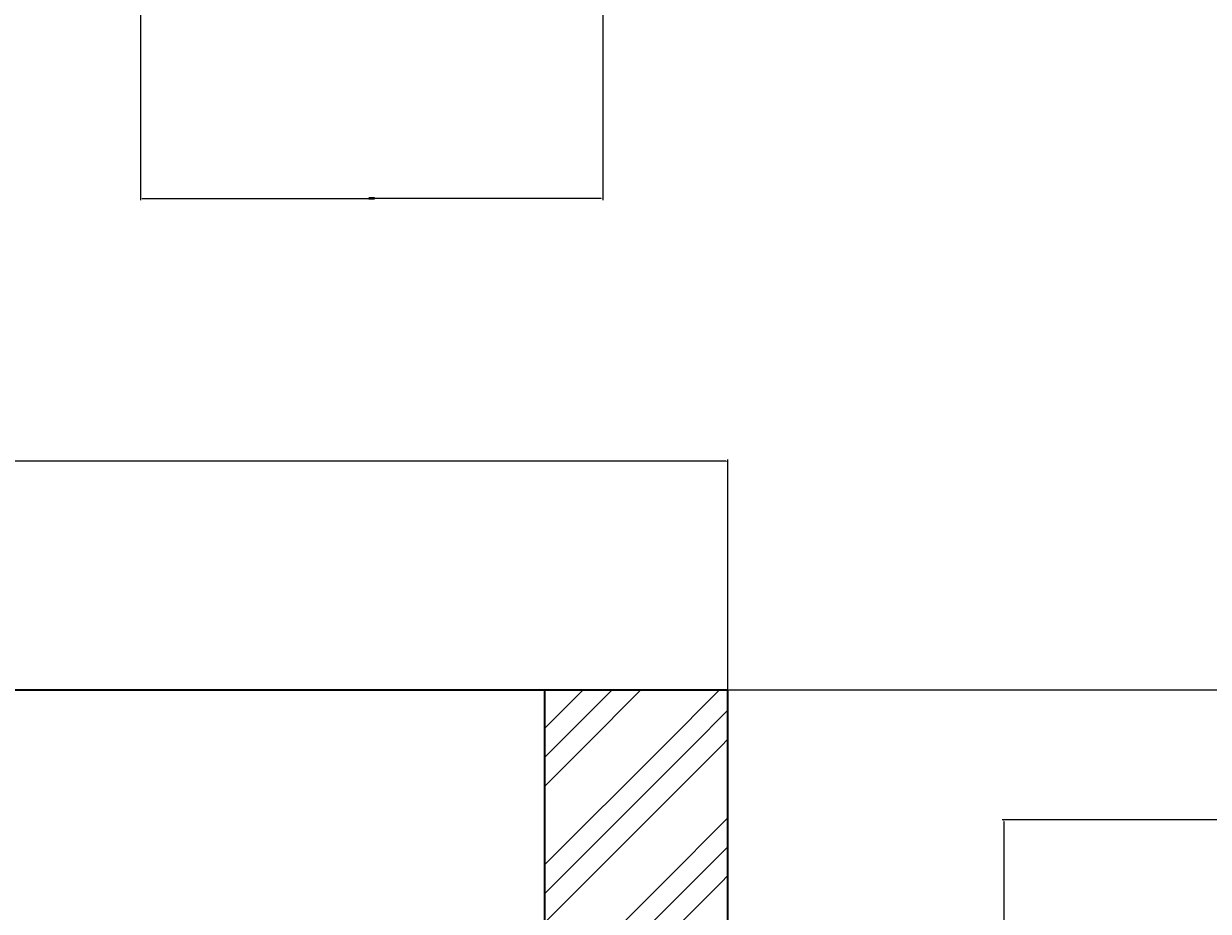
# Model space of a CAD drawing. Units: inches. Extents: x -128 to 854, y -395 to 398.
# Tile 21 of 61: x 245 to 368, y -201 to -109. Entities that reach past the tile are written whole.
import ezdxf

# ---------------------------------------------------------------- set-up
doc = ezdxf.new("R2010")
doc.units = ezdxf.units.IN
doc.header["$MEASUREMENT"] = 0
for name, color, linetype, lineweight in [('A-ANNO-DIMS', 2, 'Continuous', 18), ('A-SECT', 220, 'Continuous', 35), ('A-SECT-PATT', 8, 'Continuous', 13)]:
    doc.layers.add(name, color=color, linetype=linetype, lineweight=lineweight)
doc.styles.get("Standard").update_dxf_attribs({"font": 'arial.ttf'})
doc.dimstyles.get("Standard").update_dxf_attribs({"dimtxt": 0.18, "dimasz": 0.18, "dimexe": 0.18, "dimexo": 0.0625, "dimgap": 0.09, "dimtad": 0, "dimtih": 1, "dimtoh": 1, "dimdec": 1, "dimzin": 0, "dimdsep": 46, "dimlunit": 4, "dimtxsty": 'Standard', "dimcen": 0.09, "dimclrd": 1, "dimclre": 2, "dimclrt": 6, "dimadec": 0, "dimazin": 0, "dimtfac": 1, "dimtdec": 1, "dimtofl": 0, "dimtmove": 0, "dimatfit": 3, "dimfxl": 1, "dimtfill": 2, "dimtfillclr": 3, "dimtolj": 1, "dimtzin": 0, "dimarcsym": 0})

# ---------------------------------------------------------------- blocks, each defined once
blk = doc.blocks.new('*D114')
at = {"layer": 'A-ANNO-DIMS', "color": 2, "lineweight": -2, "transparency": 16777216}
for p, q in [((256.87, -80.32), (256.87, -127.24)), ((304.87, -80.32), (304.87, -127.24))]:
    blk.add_line(p, q, dxfattribs=at)
at = {"layer": 'A-ANNO-DIMS', "color": 1, "lineweight": -2, "transparency": 16777216}
for p, q in [((257.05, -127.06), (280.54, -127.06)), ((304.69, -127.06), (281.21, -127.06))]:
    blk.add_line(p, q, dxfattribs=at)
at = {"layer": 'A-ANNO-DIMS', "color": 1, "transparency": 16777216}
for points in [[(257.05, -127.03), (257.05, -127.09), (256.87, -127.06)], [(304.69, -127.03), (304.69, -127.09), (304.87, -127.06)]]:
    blk.add_solid(points, dxfattribs=at)
at = {"layer": 'Defpoints', "color": 0, "transparency": 16777216}
for p in [(256.87, -80.26), (304.87, -80.26), (256.87, -127.06)]:
    blk.add_point(p, dxfattribs=at)
at = {"layer": 'A-ANNO-DIMS', "color": 6, "transparency": 16777216, "insert": (280.87, -127.06), "char_height": 0.18, "attachment_point": 5, "bg_fill": 1, "box_fill_scale": 1.25, "bg_fill_color": 3, "bg_fill_transparency": 0}
blk.add_mtext('\\A1;4\'-0"', dxfattribs=at)
blk = doc.blocks.new('*D119')
at = {"layer": 'A-ANNO-DIMS', "color": 2, "lineweight": -2, "transparency": 16777216}
for p, q in [((-56.16, -177.96), (-56.16, -154.14)), ((317.84, -177.96), (317.84, -154.14))]:
    blk.add_line(p, q, dxfattribs=at)
at = {"layer": 'A-ANNO-DIMS', "color": 1, "lineweight": -2, "transparency": 16777216}
for p, q in [((-55.98, -154.32), (130.44, -154.32)), ((317.66, -154.32), (131.24, -154.32))]:
    blk.add_line(p, q, dxfattribs=at)
at = {"layer": 'A-ANNO-DIMS', "color": 1, "transparency": 16777216}
for points in [[(-55.98, -154.29), (-55.98, -154.35), (-56.16, -154.32)], [(317.66, -154.29), (317.66, -154.35), (317.84, -154.32)]]:
    blk.add_solid(points, dxfattribs=at)
at = {"layer": 'Defpoints', "color": 0, "transparency": 16777216}
for p in [(317.84, -154.32), (-56.16, -178.02), (317.84, -178.02)]:
    blk.add_point(p, dxfattribs=at)
at = {"layer": 'A-ANNO-DIMS', "color": 6, "transparency": 16777216, "insert": (130.84, -154.32), "char_height": 0.18, "attachment_point": 5, "bg_fill": 1, "box_fill_scale": 1.25, "bg_fill_color": 3, "bg_fill_transparency": 0}
blk.add_mtext('\\A1;31\'-2"', dxfattribs=at)
blk = doc.blocks.new('*D120')
at = {"layer": 'A-ANNO-DIMS', "color": 2, "lineweight": -2, "transparency": 16777216}
for p, q in [((317.9, -178.02), (389.72, -178.02)), ((337.9, -358.02), (389.72, -358.02))]:
    blk.add_line(p, q, dxfattribs=at)
at = {"layer": 'A-ANNO-DIMS', "color": 1, "lineweight": -2, "transparency": 16777216}
for p, q in [((389.54, -178.2), (389.54, -267.84)), ((389.54, -357.84), (389.54, -268.2))]:
    blk.add_line(p, q, dxfattribs=at)
at = {"layer": 'A-ANNO-DIMS', "color": 1, "transparency": 16777216}
for points in [[(389.51, -178.2), (389.57, -178.2), (389.54, -178.02)], [(389.51, -357.84), (389.57, -357.84), (389.54, -358.02)]]:
    blk.add_solid(points, dxfattribs=at)
at = {"layer": 'Defpoints', "color": 0, "transparency": 16777216}
for p in [(317.84, -178.02), (337.84, -358.02), (389.54, -358.02)]:
    blk.add_point(p, dxfattribs=at)
at = {"layer": 'A-ANNO-DIMS', "color": 6, "transparency": 16777216, "insert": (389.54, -268.02), "char_height": 0.18, "attachment_point": 5, "bg_fill": 1, "box_fill_scale": 1.25, "bg_fill_color": 3, "bg_fill_transparency": 0}
blk.add_mtext('\\A1;15\'-0"', dxfattribs=at)
blk = doc.blocks.new('*D134')
at = {"layer": 'A-ANNO-DIMS', "color": 2, "lineweight": -2, "transparency": 16777216}
for p, q in [((418.22, -191.48), (346.3, -191.48)), ((418.22, -371.48), (346.3, -371.48))]:
    blk.add_line(p, q, dxfattribs=at)
at = {"layer": 'A-ANNO-DIMS', "color": 1, "lineweight": -2, "transparency": 16777216}
for p, q in [((346.48, -191.66), (346.48, -281.29)), ((346.48, -371.3), (346.48, -281.66))]:
    blk.add_line(p, q, dxfattribs=at)
at = {"layer": 'A-ANNO-DIMS', "color": 1, "transparency": 16777216}
for points in [[(346.45, -191.66), (346.51, -191.66), (346.48, -191.48)], [(346.45, -371.3), (346.51, -371.3), (346.48, -371.48)]]:
    blk.add_solid(points, dxfattribs=at)
at = {"layer": 'Defpoints', "color": 0, "transparency": 16777216}
for p in [(346.48, -191.48), (418.28, -191.48), (418.28, -371.48)]:
    blk.add_point(p, dxfattribs=at)
at = {"layer": 'A-ANNO-DIMS', "color": 6, "transparency": 16777216, "insert": (346.48, -281.48), "char_height": 0.18, "attachment_point": 5, "bg_fill": 1, "box_fill_scale": 1.25, "bg_fill_color": 3, "bg_fill_transparency": 0}
blk.add_mtext('\\A1;15\'-0"', dxfattribs=at)

msp = doc.modelspace()

# ---------------------------------------------------------------- hatches: boundary and pattern name
at = {"layer": 'A-SECT-PATT'}
h = msp.add_hatch(dxfattribs=at)
h.set_pattern_fill('GOST_GROUND', color=256)
h.set_pattern_definition([(45, (0, 0), (14.14214, -9e-16), [20]), (45, (3, 0), (14.14214, -9e-16), [20]), (45, (6, 0), (14.14214, -9e-16), [20])])
h.paths.add_polyline_path([(-37.16, -178.02), (-56.16, -178.02), (-56.16, -202.02), (-37.16, -202.02)])
h.paths.add_polyline_path([(160.84, -178.02), (141.84, -178.02), (141.84, -202.02), (160.84, -202.02)])
h.paths.add_polyline_path([(160.84, -207.02), (141.84, -207.02), (141.84, -226.02), (160.84, -226.02)])
h.paths.add_polyline_path([(317.84, -178.02), (298.84, -178.02), (298.84, -202.02), (317.84, -202.02)])
h.paths.add_polyline_path([(317.84, -207.02), (298.84, -207.02), (298.84, -226.02), (317.84, -226.02)])
h.paths.add_polyline_path([(317.84, -274.02), (298.84, -274.02), (298.84, -298.02), (303.84, -298.02), (312.84, -298.02), (317.84, -298.02)])

# ---------------------------------------------------------------- linework, layer by layer
at = {"layer": 'A-SECT'}
for p, q in [((-56.16, -178.02), (317.84, -178.02)), ((298.84, -298.02), (298.84, -178.02)), ((317.84, -298.02), (317.84, -178.02))]:
    msp.add_line(p, q, dxfattribs=at)

# ---------------------------------------------------------------- dimensions: what is measured, and where the dimension line sits
at = {"layer": 'A-ANNO-DIMS'}
for base, p1, p2, picture, middle in [((256.87, -127.06), (304.87, -80.26), (256.87, -80.26), '*D114', (280.87, -127.06)), ((317.84, -154.32), (-56.16, -178.02), (317.84, -178.02), '*D119', (130.84, -154.32))]:
    dim = msp.add_linear_dim(base=base, p1=p1, p2=p2, dimstyle='Standard', override={"dimdec": 1, "dimlfac": 1, "dimrnd": 0, "dimzin": 1, "dimdsep": 46, "dimlunit": 4, "dimfrac": 2}, dxfattribs=at)
    dim.commit()
    dim.dimension.update_dxf_attribs({"geometry": picture, "text_midpoint": middle})
for base, p1, p2, picture, middle in [((389.54, -358.02), (317.84, -178.02), (337.84, -358.02), '*D120', (389.54, -268.02)), ((346.48, -191.48), (418.28, -371.48), (418.28, -191.48), '*D134', (346.48, -281.48))]:
    dim = msp.add_linear_dim(base=base, p1=p1, p2=p2, angle=90, dimstyle='Standard', override={"dimdec": 1, "dimlfac": 1, "dimrnd": 0, "dimzin": 1, "dimdsep": 46, "dimlunit": 4, "dimfrac": 2}, dxfattribs=at)
    dim.commit()
    dim.dimension.update_dxf_attribs({"geometry": picture, "text_midpoint": middle})

doc.saveas('drawing.dxf')
